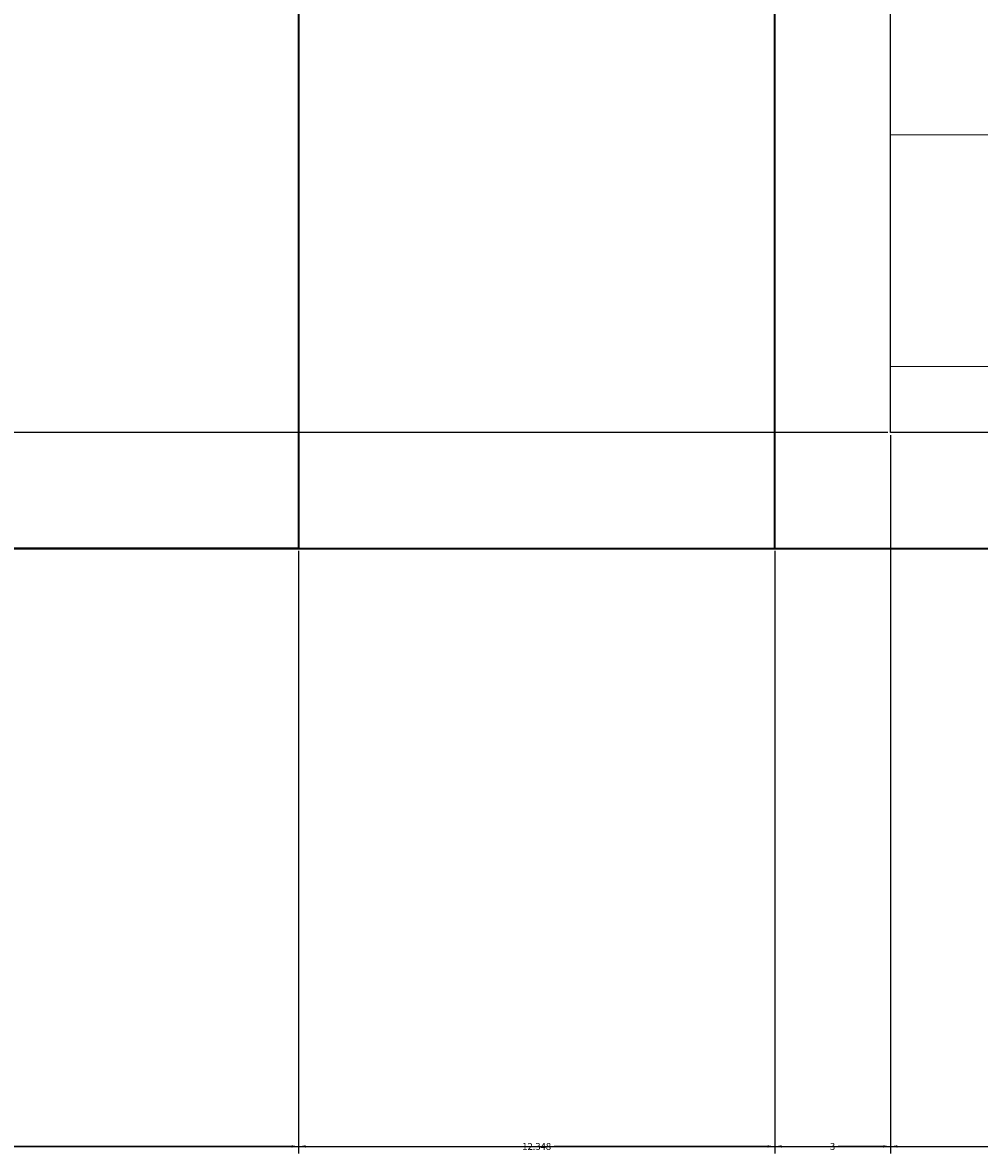
# Model space of a CAD drawing. Units: inches. Extents: x -6 to 289, y -8 to 323.
# Tile 14 of 107: x 102 to 126, y -8 to 21. Entities that reach past the tile are written whole.
import ezdxf

# ---------------------------------------------------------------- set-up
doc = ezdxf.new("R2010")
doc.units = ezdxf.units.IN
doc.header["$MEASUREMENT"] = 0
for name, color, linetype, lineweight in [('A-ANNO-DIMS', 2, 'Continuous', 18), ('A-DOOR', 3, 'Continuous', 25), ('A-ELEV', 7, 'Continuous', 35), ('A-ELEV-PATT', 8, 'Continuous', 13)]:
    doc.layers.add(name, color=color, linetype=linetype, lineweight=lineweight)
doc.styles.get("Standard").update_dxf_attribs({"font": 'arial.ttf'})
doc.dimstyles.get("Standard").update_dxf_attribs({"dimtxt": 0.18, "dimasz": 0.18, "dimexe": 0.18, "dimexo": 0.0625, "dimgap": 0.09, "dimtad": 0, "dimtih": 1, "dimtoh": 1, "dimdec": 4, "dimzin": 0, "dimdsep": 46, "dimtxsty": 'Standard', "dimcen": 0.09, "dimadec": 0, "dimazin": 0, "dimtfac": 1, "dimtdec": 4, "dimtofl": 0, "dimtmove": 0, "dimatfit": 3, "dimfxl": 1, "dimtolj": 1, "dimtzin": 0, "dimarcsym": 0})

# ---------------------------------------------------------------- blocks, each defined once
blk = doc.blocks.new('*D16')
at = {"layer": 'A-ANNO-DIMS', "color": 0, "lineweight": -2, "transparency": 16777216}
for p, q in [((9.943, 68.37), (9.943, -8.391)), ((272.973, 68.37), (272.973, -8.391)), ((10.123, -8.211), (140.993, -8.211)), ((272.793, -8.211), (141.923, -8.211))]:
    blk.add_line(p, q, dxfattribs=at)
at = {"layer": 'A-ANNO-DIMS', "color": 0, "transparency": 16777216}
for points in [[(10.123, -8.181), (10.123, -8.241), (9.943, -8.211)], [(272.793, -8.181), (272.793, -8.241), (272.973, -8.211)]]:
    blk.add_solid(points, dxfattribs=at)
at = {"layer": 'Defpoints', "color": 0, "transparency": 16777216}
for p in [(9.943, 68.432), (272.973, 68.432), (272.973, -8.211)]:
    blk.add_point(p, dxfattribs=at)
at = {"layer": 'A-ANNO-DIMS', "color": 0, "transparency": 16777216, "insert": (141.458, -8.211), "char_height": 0.18, "attachment_point": 5}
blk.add_mtext('\\A1;263.03', dxfattribs=at)
blk = doc.blocks.new('*D55')
at = {"layer": 'A-ANNO-DIMS', "color": 0, "lineweight": -2, "transparency": 16777216}
for p, q in [((92.562, 16.629), (92.562, -8.391)), ((108.66, 7.226), (108.66, -8.391)), ((92.742, -8.211), (100.156, -8.211)), ((108.48, -8.211), (101.067, -8.211))]:
    blk.add_line(p, q, dxfattribs=at)
at = {"layer": 'A-ANNO-DIMS', "color": 0, "transparency": 16777216}
for points in [[(92.742, -8.181), (92.742, -8.241), (92.562, -8.211)], [(108.48, -8.181), (108.48, -8.241), (108.66, -8.211)]]:
    blk.add_solid(points, dxfattribs=at)
at = {"layer": 'Defpoints', "color": 0, "transparency": 16777216}
for p in [(92.562, 16.692), (108.66, 7.289), (108.66, -8.211)]:
    blk.add_point(p, dxfattribs=at)
at = {"layer": 'A-ANNO-DIMS', "color": 0, "transparency": 16777216, "insert": (100.611, -8.211), "char_height": 0.18, "attachment_point": 5}
blk.add_mtext('\\A1;16.098', dxfattribs=at)
blk = doc.blocks.new('*D56')
at = {"layer": 'A-ANNO-DIMS', "color": 0, "lineweight": -2, "transparency": 16777216}
for p, q in [((108.66, 7.226), (108.66, -8.391)), ((121.008, 7.226), (121.008, -8.391)), ((108.84, -8.211), (114.379, -8.211)), ((120.828, -8.211), (115.289, -8.211))]:
    blk.add_line(p, q, dxfattribs=at)
at = {"layer": 'A-ANNO-DIMS', "color": 0, "transparency": 16777216}
for points in [[(108.84, -8.181), (108.84, -8.241), (108.66, -8.211)], [(120.828, -8.181), (120.828, -8.241), (121.008, -8.211)]]:
    blk.add_solid(points, dxfattribs=at)
at = {"layer": 'Defpoints', "color": 0, "transparency": 16777216}
for p in [(108.66, 7.289), (121.008, 7.289), (121.008, -8.211)]:
    blk.add_point(p, dxfattribs=at)
at = {"layer": 'A-ANNO-DIMS', "color": 0, "transparency": 16777216, "insert": (114.834, -8.211), "char_height": 0.18, "attachment_point": 5}
blk.add_mtext('\\A1;12.348', dxfattribs=at)
blk = doc.blocks.new('*D67')
at = {"layer": 'A-ANNO-DIMS', "color": 0, "lineweight": -2, "transparency": 16777216}
for p, q in [((124.008, 10.226), (124.008, -8.391)), ((121.008, 7.226), (121.008, -8.391)), ((121.188, -8.211), (122.359, -8.211)), ((123.828, -8.211), (122.657, -8.211))]:
    blk.add_line(p, q, dxfattribs=at)
at = {"layer": 'A-ANNO-DIMS', "color": 0, "transparency": 16777216}
for points in [[(121.188, -8.181), (121.188, -8.241), (121.008, -8.211)], [(123.828, -8.181), (123.828, -8.241), (124.008, -8.211)]]:
    blk.add_solid(points, dxfattribs=at)
at = {"layer": 'Defpoints', "color": 0, "transparency": 16777216}
for p in [(124.008, 10.289), (121.008, 7.289), (124.008, -8.211)]:
    blk.add_point(p, dxfattribs=at)
at = {"layer": 'A-ANNO-DIMS', "color": 0, "transparency": 16777216, "insert": (122.508, -8.211), "char_height": 0.18, "attachment_point": 5}
blk.add_mtext('\\A1;3', dxfattribs=at)
blk = doc.blocks.new('*D68')
at = {"layer": 'A-ANNO-DIMS', "color": 0, "lineweight": -2, "transparency": 16777216}
for p, q in [((124.008, 10.226), (124.008, -8.391)), ((184.124, 10.226), (184.124, -8.391)), ((124.188, -8.211), (153.673, -8.211)), ((183.944, -8.211), (154.459, -8.211))]:
    blk.add_line(p, q, dxfattribs=at)
at = {"layer": 'A-ANNO-DIMS', "color": 0, "transparency": 16777216}
for points in [[(124.188, -8.181), (124.188, -8.241), (124.008, -8.211)], [(183.944, -8.181), (183.944, -8.241), (184.124, -8.211)]]:
    blk.add_solid(points, dxfattribs=at)
at = {"layer": 'Defpoints', "color": 0, "transparency": 16777216}
for p in [(124.008, 10.289), (184.124, 10.289), (184.124, -8.211)]:
    blk.add_point(p, dxfattribs=at)
at = {"layer": 'A-ANNO-DIMS', "color": 0, "transparency": 16777216, "insert": (154.066, -8.211), "char_height": 0.18, "attachment_point": 5}
blk.add_mtext('\\A1;60.12', dxfattribs=at)
blk = doc.blocks.new('*D83')
at = {"layer": 'A-ANNO-DIMS', "color": 0, "lineweight": -2, "transparency": 16777216}
for p, q in [((123.945, 10.289), (-5.737, 10.289)), ((-5.557, 10.109), (-5.557, 8.971)), ((-5.557, 7.469), (-5.557, 8.607)), ((120.945, 7.289), (-5.737, 7.289))]:
    blk.add_line(p, q, dxfattribs=at)
at = {"layer": 'A-ANNO-DIMS', "color": 0, "transparency": 16777216}
for points in [[(-5.587, 10.109), (-5.527, 10.109), (-5.557, 10.289)], [(-5.587, 7.469), (-5.527, 7.469), (-5.557, 7.289)]]:
    blk.add_solid(points, dxfattribs=at)
at = {"layer": 'Defpoints', "color": 0, "transparency": 16777216}
for p in [(-5.557, 10.289), (124.008, 10.289), (121.008, 7.289)]:
    blk.add_point(p, dxfattribs=at)
at = {"layer": 'A-ANNO-DIMS', "color": 0, "transparency": 16777216, "insert": (-5.557, 8.789), "char_height": 0.18, "attachment_point": 5}
blk.add_mtext('\\A1;3', dxfattribs=at)
blk = doc.blocks.new('*D84')
at = {"layer": 'A-ANNO-DIMS', "color": 0, "lineweight": -2, "transparency": 16777216}
for p, q in [((123.945, 48.085), (-5.737, 48.085)), ((-5.557, 47.905), (-5.557, 29.369)), ((-5.557, 10.469), (-5.557, 29.005)), ((123.945, 10.289), (-5.737, 10.289))]:
    blk.add_line(p, q, dxfattribs=at)
at = {"layer": 'A-ANNO-DIMS', "color": 0, "transparency": 16777216}
for points in [[(-5.587, 47.905), (-5.527, 47.905), (-5.557, 48.085)], [(-5.587, 10.469), (-5.527, 10.469), (-5.557, 10.289)]]:
    blk.add_solid(points, dxfattribs=at)
at = {"layer": 'Defpoints', "color": 0, "transparency": 16777216}
for p in [(-5.557, 48.085), (124.008, 48.085), (124.008, 10.289)]:
    blk.add_point(p, dxfattribs=at)
at = {"layer": 'A-ANNO-DIMS', "color": 0, "transparency": 16777216, "insert": (-5.557, 29.187), "char_height": 0.18, "attachment_point": 5}
blk.add_mtext('\\A1;37.8', dxfattribs=at)

msp = doc.modelspace()

# ---------------------------------------------------------------- hatches: boundary and pattern name
at = {"layer": 'A-ELEV-PATT'}
h = msp.add_hatch(dxfattribs=at)
h.set_pattern_fill('_USER', color=256, scale=6, pattern_type=0)
h.set_pattern_definition([(0, (0, 0), (0, 6), [])])
h.paths.add_polyline_path([(184.1244, 48.0851), (124.008, 48.0851), (124.008, 10.2888), (184.1244, 10.2888)])
h.paths.add_polyline_path([(244.2408, 48.0851), (186.3604, 48.0851), (186.3604, 10.2888), (244.2408, 10.2888)])
h.paths.add_polyline_path([(208.2918, 114.2795), (190.7918, 114.2795), (190.7918, 71.2795), (208.2918, 71.2795)])
h.paths.add_polyline_path([(227.7918, 114.2795), (209.2918, 114.2795), (209.2918, 71.2795), (227.7918, 71.2795)])
h.paths.add_polyline_path([(211.2918, 224.3887), (190.7918, 224.3887), (190.7918, 162.3484), (211.2918, 162.3484)])
h.paths.add_polyline_path([(233.7918, 224.3887), (212.2918, 224.3887), (212.2918, 162.3484), (233.7918, 162.3484)])
h.paths.add_polyline_path([(166.3835, 224.154), (147.8835, 224.154), (147.8835, 181.154), (166.3835, 181.154)])
h.paths.add_polyline_path([(146.8835, 224.154), (129.3835, 224.154), (129.3835, 181.154), (146.8835, 181.154)])

# ---------------------------------------------------------------- linework, layer by layer
at = {"layer": 'A-DOOR'}
for points in [[(121.008, 51.0851), (247.2408, 51.0851), (247.2408, 7.2888), (121.008, 7.2888)], [(124.008, 48.0851), (244.2408, 48.0851), (244.2408, 10.2888), (124.008, 10.2888)]]:
    msp.add_lwpolyline(points, close=True, dxfattribs=at)
at = {"layer": 'A-ELEV'}
msp.add_line((19.1638, 7.2888), (271.1638, 7.2888), dxfattribs=at)
msp.add_lwpolyline([(108.6602, 66.2238), (108.6602, 7.2888), (121.008, 7.2888), (121.008, 66.2238)], dxfattribs=at)
msp.add_lwpolyline([(24.317, 49.3604), (108.6602, 49.3604), (108.6602, 7.2888), (24.317, 7.2888)], close=True, dxfattribs=at)

# ---------------------------------------------------------------- dimensions: what is measured, and where the dimension line sits
at = {"layer": 'A-ANNO-DIMS'}
for base, p1, p2, override, picture, middle in [((272.9733, -8.2112), (9.943, 68.4322), (272.9733, 68.4322), {"dimdec": 2, "dimlfac": 1, "dimrnd": 0, "dimzin": 0, "dimdsep": 46, "dimlunit": 2}, '*D16', (141.4581, -8.2112)), ((108.6602, -8.2112), (92.5623, 16.6917), (108.6602, 7.2888), {"dimdec": 3, "dimlfac": 1, "dimrnd": 0, "dimzin": 0, "dimdsep": 46, "dimlunit": 2}, '*D55', (100.6113, -8.2112)), ((124.008, -8.2112), (121.008, 7.2888), (124.008, 10.2888), {"dimdec": 0, "dimlfac": 1, "dimrnd": 0, "dimzin": 0, "dimdsep": 46, "dimlunit": 2}, '*D67', (122.508, -8.2112)), ((184.1244, -8.2112), (124.008, 10.2888), (184.1244, 10.2888), {"dimdec": 2, "dimlfac": 1, "dimrnd": 0, "dimzin": 0, "dimdsep": 46, "dimlunit": 2}, '*D68', (154.0662, -8.2112)), ((121.008, -8.2112), (108.6602, 7.2888), (121.008, 7.2888), {"dimdec": 3, "dimlfac": 1, "dimrnd": 0, "dimzin": 0, "dimdsep": 46, "dimlunit": 2}, '*D56', (114.8341, -8.2112))]:
    dim = msp.add_linear_dim(base=base, p1=p1, p2=p2, dimstyle='Standard', override=override, dxfattribs=at)
    dim.commit()
    dim.dimension.update_dxf_attribs({"geometry": picture, "text_midpoint": middle})
for base, p1, p2, override, picture, middle in [((-5.557, 48.0851), (124.008, 10.2888), (124.008, 48.0851), {"dimdec": 1, "dimlfac": 1, "dimrnd": 0, "dimzin": 0, "dimdsep": 46, "dimlunit": 2}, '*D84', (-5.557, 29.187)), ((-5.557, 10.2888), (121.008, 7.2888), (124.008, 10.2888), {"dimdec": 0, "dimlfac": 1, "dimrnd": 0, "dimzin": 0, "dimdsep": 46, "dimlunit": 2}, '*D83', (-5.557, 8.7888))]:
    dim = msp.add_linear_dim(base=base, p1=p1, p2=p2, angle=90, dimstyle='Standard', override=override, dxfattribs=at)
    dim.commit()
    dim.dimension.update_dxf_attribs({"geometry": picture, "text_midpoint": middle})

doc.saveas('drawing.dxf')
